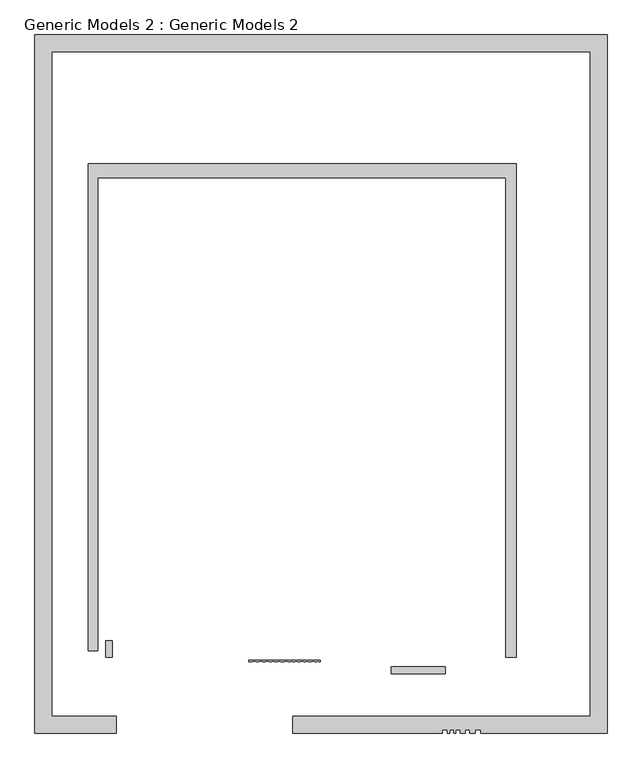
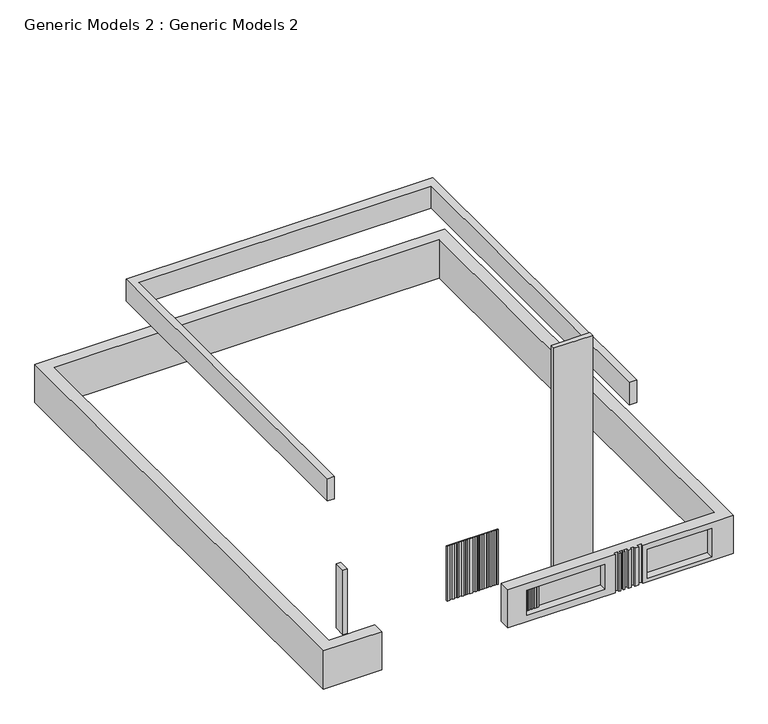
"""IFC4 building model written with IfcOpenShell, lengths in millimetres: proxy geometry, Generic Models 2 : Generic Models 2."""

from ifc_helpers import new_model, si_unit, frame, origin, origin_with_axes, place, context, project, spatial, polyline, outline, extrude, faceted_brep, source, transform, mapped, element, save


def generic_models_2_generic_models_2_9e54925f(model_context):
    return source(origin(), model_context, "Body", "SolidModel", [
        extrude(outline(polyline([(-4213.0047537, -21109.0428796), (-4543.2047537, -21109.0428796), (-4543.2047537, -5754.7428796), (-17624.2047537, -5754.7428796), (-17624.2047537, -20896.5943683), (-17929.0047537, -20896.5943683), (-17929.0047537, -5297.5428796), (-4213.0047537, -5297.5428796), (-4213.0047537, -21109.0428796)])), frame((0.0, 0.0, 6400.8), z_axis=(0.0, 0.0, 1.0), x_axis=(1.0, 0.0, 0.0)), (0.0, 0.0, 1.0), 1051.1676894),
        extrude(outline(polyline([(-17156.3088717, -21109.0428796), (-17357.5047537, -21109.0428796), (-17357.5047537, -20588.6333933), (-17156.3088717, -20588.6333933), (-17156.3088717, -21109.0428796)])), origin_with_axes(), (0.0, 0.0, 1.0), 3048.0),
        extrude(outline(polyline([(-10373.3771758, -23287.4611591), (-10443.9515861, -23287.4611591), (-10443.9515861, -23185.8611591), (-10373.3771758, -23185.8611591), (-10373.3771758, -23287.4611591)])), origin_with_axes(), (0.0, 0.0, 1.0), 1187.9248474),
        extrude(outline(polyline([(-10249.9467739, -23287.4611591), (-10324.005015, -23287.4611591), (-10324.005015, -23185.8611591), (-10249.9467739, -23185.8611591), (-10249.9467739, -23287.4611591)])), origin_with_axes(), (0.0, 0.0, 1.0), 1187.9248474),
        extrude(outline(polyline([(-10118.2876786, -23287.4611591), (-10192.3459197, -23287.4611591), (-10192.3459197, -23185.8611591), (-10118.2876786, -23185.8611591), (-10118.2876786, -23287.4611591)])), origin_with_axes(), (0.0, 0.0, 1.0), 1187.9248474),
        extrude(outline(polyline([(-9966.1047537, -23287.4611591), (-10052.4581309, -23287.4611591), (-10052.4581309, -23185.8611591), (-9966.1047537, -23185.8611591), (-9966.1047537, -23287.4611591)])), origin_with_axes(), (0.0, 0.0, 1.0), 1187.9248474),
        extrude(outline(polyline([(-9851.8047537, -23287.4611591), (-9916.6846889, -23287.4611591), (-9916.6846889, -23185.8611591), (-9851.8047537, -23185.8611591), (-9851.8047537, -23287.4611591)])), origin_with_axes(), (0.0, 0.0, 1.0), 1187.9248474),
        faceted_brep([(-19632.6714631, -23541.4611591, -304.8), (-19632.6714631, -23541.4611591, 1498.4935587), (-19632.6714631, -1170.4008704, 1498.4935587), (-19632.6714631, -1170.4008704, -304.8), (-19099.2714631, -23008.0611591, -304.8), (-19099.2714631, -1703.8008704, -304.8), (-19099.2714631, -1703.8008704, 1498.4935587), (-19099.2714631, -23008.0611591, 1498.4935587), (-17031.755135, -23008.0611591, 1498.4935587), (-1831.4052444, -1703.8008704, 1498.4935587), (-1831.4052444, -23008.0611591, 1498.4935587), (-11375.8047537, -23008.0611591, 1498.4935587), (-11375.8047537, -23541.4611591, 1498.4935587), (-6580.2045866, -23541.4611591, 1498.4935587), (-6580.2045866, -23439.8611591, 1498.4935587), (-6424.0857737, -23439.8611591, 1498.4935587), (-6424.0857737, -23541.4611591, 1498.4935587), (-6336.9049991, -23541.4611591, 1498.4935587), (-6336.9049991, -23439.8611591, 1498.4935587), (-6209.0710712, -23439.8611591, 1498.4935587), (-6209.0710712, -23541.4611591, 1498.4935587), (-6144.5001374, -23541.4611591, 1498.4935587), (-6144.5001374, -23439.8611591, 1498.4935587), (-5998.4514718, -23439.8611591, 1498.4935587), (-5998.4514718, -23541.4611591, 1498.4935587), (-5847.5982082, -23541.4611591, 1498.4935587), (-5847.5982082, -23439.8611591, 1498.4935587), (-5704.3617833, -23439.8611591, 1498.4935587), (-5704.3617833, -23541.4611591, 1498.4935587), (-5529.1754263, -23541.4611591, 1498.4935587), (-5529.1754263, -23439.8611591, 1498.4935587), (-5341.0165097, -23439.8611591, 1498.4935587), (-5341.0165097, -23541.4611591, 1498.4935587), (-1298.0052444, -23541.4611591, 1498.4935587), (-1298.0052444, -1170.4008704, 1498.4935587), (-17031.755135, -23541.4611591, 1498.4935587), (-17031.755135, -23008.0611591, -304.8), (-17031.755135, -23541.4611591, -304.8), (-1298.0052444, -1170.4008704, -304.8), (-1298.0052444, -23541.4611591, -304.8), (-5341.0165097, -23541.4611591, -304.8), (-5341.0165097, -23439.8611591, -304.8), (-5529.1754263, -23439.8611591, -304.8), (-5529.1754263, -23541.4611591, -304.8), (-5704.3617833, -23541.4611591, -304.8), (-5704.3617833, -23439.8611591, -304.8), (-5847.5982082, -23439.8611591, -304.8), (-5847.5982082, -23541.4611591, -304.8), (-5998.4514718, -23541.4611591, -304.8), (-5998.4514718, -23439.8611591, -304.8), (-6144.5001374, -23439.8611591, -304.8), (-6144.5001374, -23541.4611591, -304.8), (-6209.0710712, -23541.4611591, -304.8), (-6209.0710712, -23439.8611591, -304.8), (-6336.9049991, -23439.8611591, -304.8), (-6336.9049991, -23541.4611591, -304.8), (-6424.0857737, -23541.4611591, -304.8), (-6424.0857737, -23439.8611591, -304.8), (-6580.2045866, -23439.8611591, -304.8), (-6580.2045866, -23541.4611591, -304.8), (-11375.8047537, -23541.4611591, -304.8), (-11375.8047537, -23008.0611591, -304.8), (-1831.4052444, -23008.0611591, -304.8), (-1831.4052444, -1703.8008704, -304.8), (-5142.4582415, -23541.4611591, -140.6932371), (-5142.4582415, -23541.4611591, 1230.9067629), (-2246.8582415, -23541.4611591, 1230.9067629), (-2246.8582415, -23541.4611591, -140.6932371), (-10538.2233692, -23541.4611591, 0.0), (-10538.2233692, -23541.4611591, 1187.9248474), (-7032.4047537, -23541.4611591, 1187.9248474), (-7032.4047537, -23541.4611591, 0.0), (-5142.4582415, -23185.8611591, -140.6932371), (-2246.8582415, -23185.8611591, -140.6932371), (-2246.8582415, -23185.8611591, 1230.9067629), (-5142.4582415, -23185.8611591, 1230.9067629), (-10538.2233692, -23185.8611591, 0.0), (-7032.4047537, -23185.8611591, 0.0), (-7032.4047537, -23185.8611591, 1187.9248474), (-10538.2233692, -23185.8611591, 1187.9248474)], [[[0, 1, 2, 3]], [[4, 5, 6, 7]], [[8, 7, 6, 9, 10, 11, 12, 13, 14, 15, 16, 17, 18, 19, 20, 21, 22, 23, 24, 25, 26, 27, 28, 29, 30, 31, 32, 33, 34, 2, 1, 35]], [[4, 36, 37, 0, 3, 38, 39, 40, 41, 42, 43, 44, 45, 46, 47, 48, 49, 50, 51, 52, 53, 54, 55, 56, 57, 58, 59, 60, 61, 62, 63, 5]], [[1, 0, 37, 35]], [[7, 8, 36, 4]], [[35, 37, 36, 8]], [[3, 2, 34, 38]], [[5, 63, 9, 6]], [[39, 38, 34, 33]], [[9, 63, 62, 10]], [[44, 43, 29, 28]], [[48, 47, 25, 24]], [[52, 51, 21, 20]], [[56, 55, 17, 16]], [[39, 33, 32, 40], [64, 65, 66, 67]], [[12, 60, 59, 13], [68, 69, 70, 71]], [[62, 61, 11, 10]], [[60, 12, 11, 61]], [[72, 73, 74, 75]], [[72, 75, 65, 64]], [[75, 74, 66, 65]], [[74, 73, 67, 66]], [[73, 72, 64, 67]], [[41, 31, 30, 42]], [[45, 27, 26, 46]], [[49, 23, 22, 50]], [[53, 19, 18, 54]], [[57, 15, 14, 58]], [[42, 30, 29, 43]], [[31, 41, 40, 32]], [[46, 26, 25, 47]], [[27, 45, 44, 28]], [[50, 22, 21, 51]], [[23, 49, 48, 24]], [[54, 18, 17, 55]], [[19, 53, 52, 20]], [[58, 14, 13, 59]], [[15, 57, 56, 16]], [[76, 77, 78, 79]], [[76, 79, 69, 68]], [[79, 78, 70, 69]], [[78, 77, 71, 70]], [[77, 76, 68, 71]]]),
        extrude(outline(polyline([(-12780.5111772, -21210.6428796), (-10494.5111772, -21210.6428796), (-10494.5111772, -21261.4428796), (-10531.889851, -21261.4428796), (-10531.889851, -21236.0428796), (-10597.4741716, -21236.0428796), (-10597.4741716, -21261.4428796), (-10664.8276401, -21261.4428796), (-10664.8276401, -21236.0428796), (-10773.652111, -21236.0428796), (-10773.652111, -21261.4428796), (-10849.8292407, -21261.4428796), (-10849.8292407, -21236.0428796), (-10947.7712646, -21236.0428796), (-10947.7712646, -21261.4428796), (-11013.0659472, -21261.4428796), (-11013.0659472, -21236.0428796), (-11132.7728652, -21236.0428796), (-11132.7728652, -21261.4428796), (-11203.5087714, -21261.4428796), (-11203.5087714, -21236.0428796), (-11312.3332424, -21236.0428796), (-11312.3332424, -21261.4428796), (-11375.8047537, -21261.4428796), (-11375.8047537, -21236.0428796), (-11456.0337981, -21236.0428796), (-11456.0337981, -21261.4428796), (-11519.7837553, -21261.4428796), (-11519.7837553, -21236.0428796), (-11637.5111772, -21236.0428796), (-11637.5111772, -21261.4428796), (-11762.19448, -21261.4428796), (-11762.19448, -21236.0428796), (-11874.8278075, -21236.0428796), (-11874.8278075, -21261.4428796), (-11949.9166925, -21261.4428796), (-11949.9166925, -21236.0428796), (-12043.7777987, -21236.0428796), (-12043.7777987, -21261.4428796), (-12125.1240907, -21261.4428796), (-12125.1240907, -21236.0428796), (-12250.2722324, -21236.0428796), (-12250.2722324, -21261.4428796), (-12337.8759315, -21261.4428796), (-12337.8759315, -21236.0428796), (-12463.0240731, -21236.0428796), (-12463.0240731, -21261.4428796), (-12545.0563334, -21261.4428796), (-12545.0563334, -21236.0428796), (-12670.1368542, -21236.0428796), (-12670.1368542, -21261.4428796), (-12780.5111772, -21261.4428796), (-12780.5111772, -21210.6428796)])), frame((0.0, 0.0, 79.8635088), z_axis=(0.0, 0.0, 1.0), x_axis=(1.0, 0.0, 0.0)), (0.0, 0.0, 1.0), 2590.8),
        extrude(outline(polyline([(-6478.9006991, -21642.4428796), (-8218.7383708, -21642.4428796), (-8218.7383708, -21413.8428796), (-6478.9006991, -21413.8428796), (-6478.9006991, -21642.4428796)])), origin_with_axes(), (0.0, 0.0, 1.0), 10690.4702873),
    ])


if __name__ == "__main__":
    model = new_model("IFC4")
    model_context = context("Model", 3, world=origin())
    ifc_project = project(units=[si_unit("LENGTHUNIT", "METRE", prefix="MILLI")], contexts=[model_context])
    site = spatial("IfcSite", under=ifc_project)
    building = spatial("IfcBuilding", under=site)
    placement = place(None, origin())
    generic_models_2_generic_models_2_shape = generic_models_2_generic_models_2_9e54925f(model_context)
    element("IfcBuildingElementProxy", 1, Name="Generic Models 2 : Generic Models 2", ObjectType="Generic Models 2 : Generic Models 2", at=placement, inside=building, context=model_context, shape_type="MappedRepresentation", body=[
        mapped(generic_models_2_generic_models_2_shape, transform((0.0, 0.0, 0.0), x_axis=(1.0, 0.0, 0.0), y_axis=(0.0, 1.0, 0.0), z_axis=(0.0, 0.0, 1.0))),
    ])
    save(model, "model.ifc")
